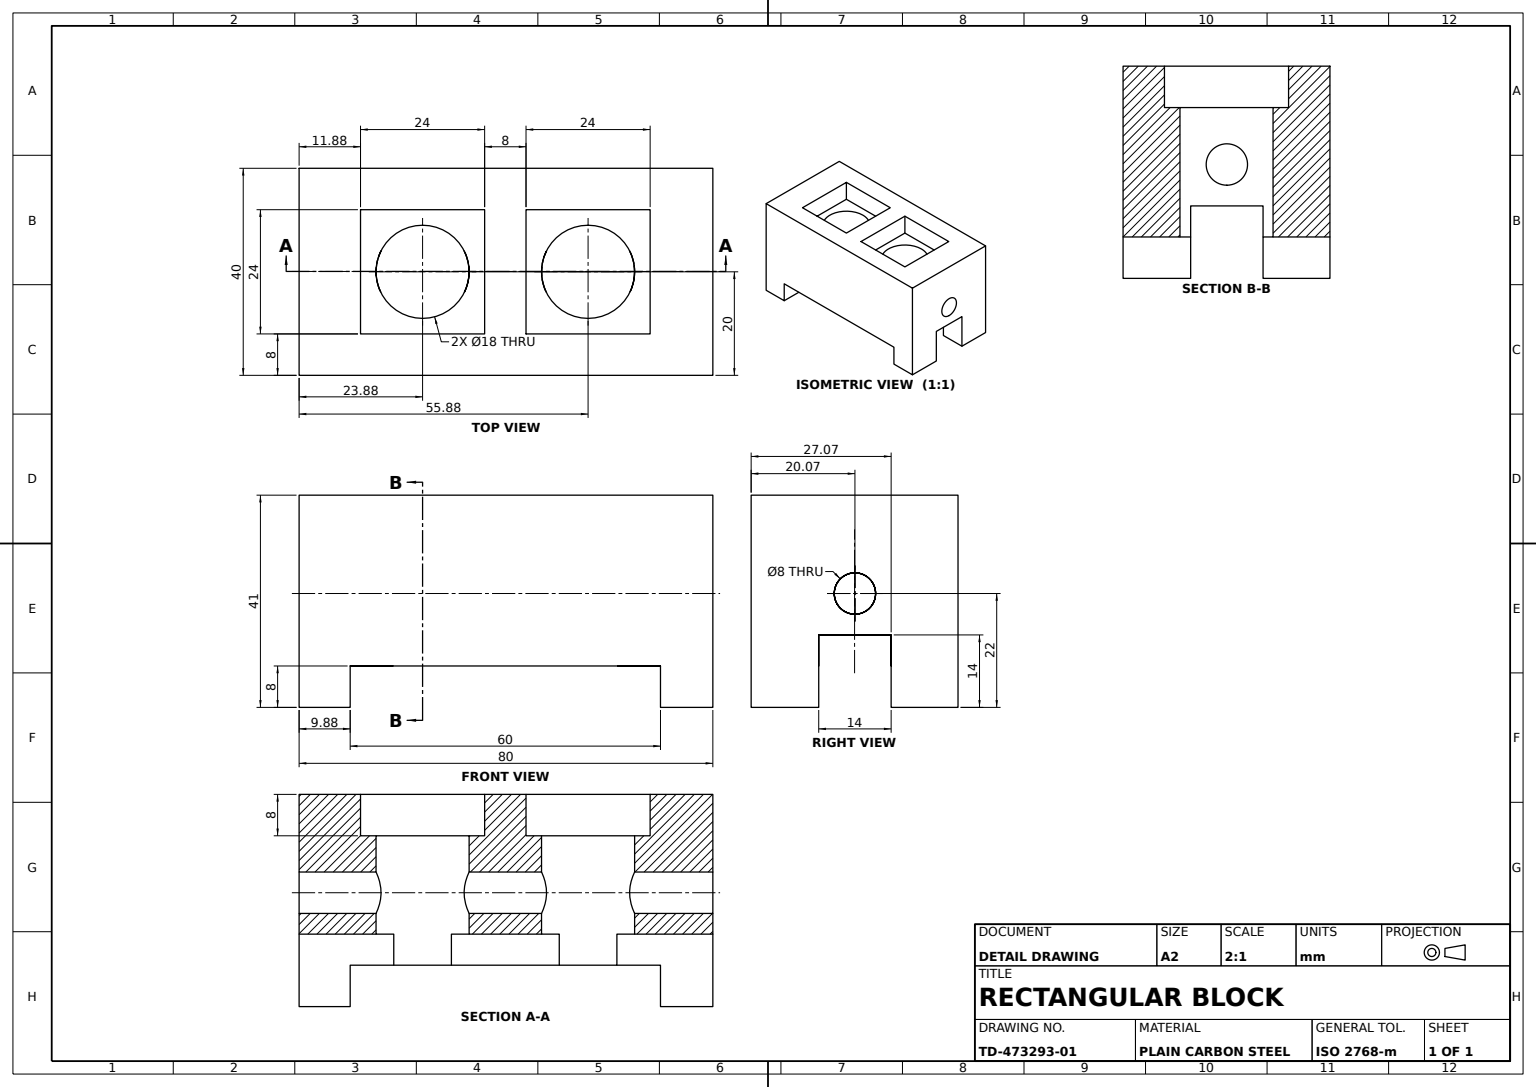
SolidWorks part; units mm, degrees
material "Plain Carbon Steel"
ref_plane "Front Plane" through (0, 0, 0) normal (0, 0, 1) x (1, 0, 0)
ref_plane "Top Plane" through (0, 0, 0) normal (0, 1, 0) x (1, 0, 0)
ref_plane "Right Plane" through (0, 0, 0) normal (1, 0, 0) x (0, 0, -1)
sketch "Block Profile Sketch" plane through (0, 0, 0) normal (0, 0, 1) x (1, 0, 0)
  line L0 (-30, 0) -> (30, 0)
  line L1 (-30, 0) -> (-30, -8)
  line L2 (-30, -8) -> (-39.875, -8)
  line L3 (-39.875, -8) -> (-39.875, 33)
  line L4 (-39.875, 33) -> (40.125, 33)
  line L5 (40.125, 33) -> (40.125, -8)
  line L6 (40.125, -8) -> (30, -8)
  line L7 (30, -8) -> (30, 0)
  point P4 (0, 0)
  dimension "D1" = 60
  dimension "D2" = 8
  dimension "D3" = 8
  dimension "D4" = 80
  dimension "D5" = 41
  dimension "D6" = 41
  dimension "D7" = 39.875
extrude "Base Block 40" add sketch "Block Profile Sketch" against normal blind 40
sketch "Square Pockets Sketch" plane through (0, 33, 0) normal (0, 1, 0) x (1, 0, 0)
  line L0 (0, -22) -> (0, 22) construction
  line L2 (40.125, 0) -> (-39.875, 0) construction
  line L3 (-28, 8) -> (-4, 8)
  line L4 (-28, 8) -> (-28, 32)
  line L5 (-28, 32) -> (-4, 32)
  line L6 (-4, 8) -> (-4, 32)
  line L7 (-39.875, 40) -> (-39.875, 0) construction
  line L8 (4, 8) -> (4, 32)
  line L9 (28, 32) -> (4, 32)
  line L10 (28, 8) -> (28, 32)
  line L11 (28, 8) -> (4, 8)
  dimension "D1" = 24
  dimension "D2" = 24
  dimension "D3" = 11.875
  dimension "D4" = 8
  dimension "D5" = 8
extrude "Square Pockets 2x24x24" cut sketch "Square Pockets Sketch" against normal blind 8
sketch "Pocket Holes Sketch" plane through (0, 25, 0) normal (0, 1, 0) x (1, 0, 0)
  line L1 (-4, 8) -> (-4, 32) construction
  line L2 (-28, 8) -> (-4, 8) construction
  line L3 (0, -22) -> (0, 22) construction
  circle A0 centre (-16, 20) radius 9
  circle A1 centre (16, 20) radius 9
  dimension "D3" = 18
  dimension "D1" = 12
  dimension "D2" = 12
extrude "Pocket Holes 2xØ12" cut sketch "Pocket Holes Sketch" against normal through all
sketch "End Bore and Slot Sketch" plane through (40.125, 0, 0) normal (1, 0, 0) x (0, 0, -1)
  line L0 (13.0675, 6) -> (27.0675, 6)
  line L1 (27.0675, 6) -> (27.0675, -8)
  line L2 (40, -8) -> (0, -8) construction
  line L3 (27.0675, -8) -> (13.0675, -8)
  line L4 (13.0675, -8) -> (13.0675, 6)
  line L5 (0, -8) -> (0, 33) construction
  circle A0 centre (20.0675, 14) radius 4
  point P3 (20.0675, 6)
  dimension "D3" = 8
  dimension "D1" = 14
  dimension "D2" = 14
  dimension "D4" = 22
  dimension "D5" = 27.0675
  dimension "D6" = 7
  dimension "D7" = 22
extrude "End Bore and Slot" cut sketch "End Bore and Slot Sketch" against normal through all
